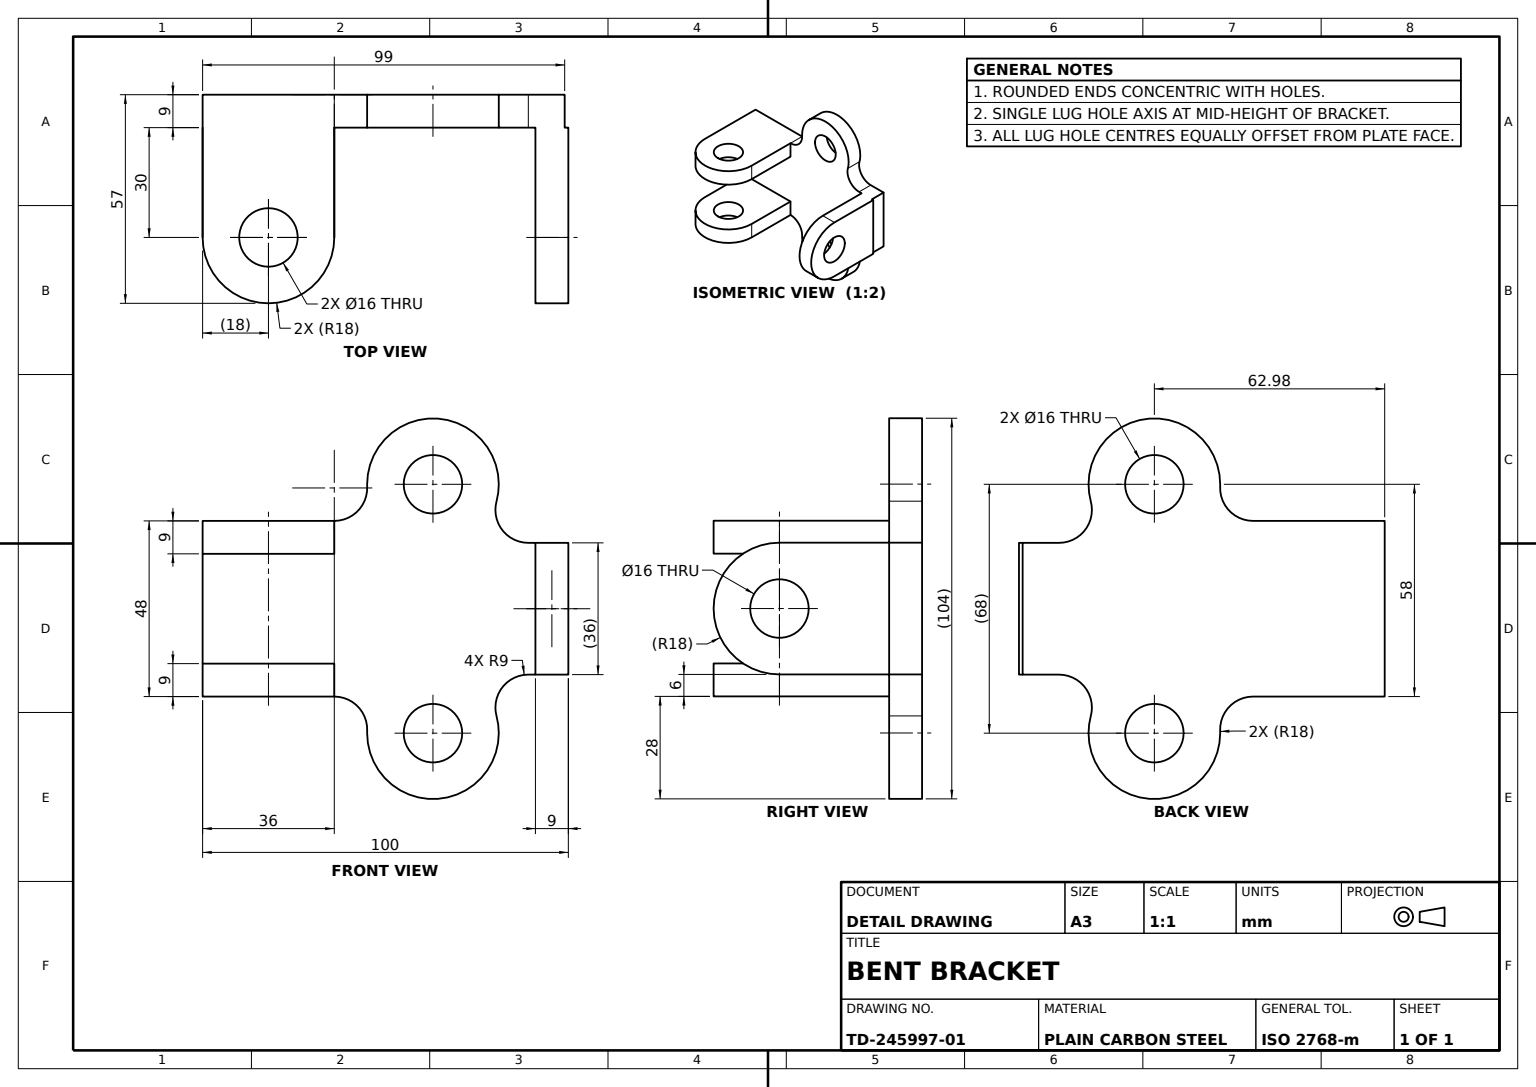
SolidWorks part; units mm, degrees
material "Plain Carbon Steel"
ref_plane "Front Plane" through (0, 0, 0) normal (0, 0, 1) x (1, 0, 0)
ref_plane "Top Plane" through (0, 0, 0) normal (0, 1, 0) x (1, 0, 0)
ref_plane "Right Plane" through (0, 0, 0) normal (1, 0, 0) x (0, 0, -1)
sketch "Base Plate Profile Sketch" plane through (0, 0, 0) normal (0, 0, 1) x (1, 0, 0)
  line L0 (0, 0) -> (0, 48)
  line L1 (0, 24) -> (62.9815, 24) construction
  line L2 (62.9815, 24) -> (99, 24) construction
  line L3 (99, 24) -> (99, 42)
  line L4 (99, 24) -> (99, 6)
  line L5 (62.9815, 24) -> (62.9815, 58) construction
  line L6 (62.9815, 24) -> (62.9815, -10) construction
  line L7 (0, 48) -> (36, 48)
  line L8 (99, 42) -> (89.0583, 42)
  line L9 (0, 0) -> (36, 0)
  line L10 (99, 6) -> (89.0583, 6)
  circle A0 centre (62.9815, 58) radius 8
  arc A1 (80.366, 53.3333) -> (44.9938, 57.3333) centre (62.9815, 58) ccw
  arc A2 (36, 48) -> (44.9938, 57.3333) centre (36, 57) ccw
  arc A3 (80.366, 53.3333) -> (89.0583, 42) centre (89.0583, 51) ccw
  circle A4 centre (62.9815, -10) radius 8
  arc A5 (44.9938, -9.3333) -> (80.366, -5.3333) centre (62.9815, -10) ccw
  arc A8 (44.9938, -9.3333) -> (36, 0) centre (36, -9) ccw
  arc A9 (89.0583, 6) -> (80.366, -5.3333) centre (89.0583, -3) ccw
  dimension "D1" = 16
  dimension "D2" = 36
  dimension "D3" = 48
  dimension "D7" = 9
  dimension "D8" = 58
  dimension "D10" = 9
  dimension "D11" = 99
  dimension "D12" = 16
  dimension "D13" = 18
  dimension "D14" = 9
  dimension "D4" = 18
  dimension "D15" = 18
  dimension "D5" = 36
  dimension "D6" = 68
  dimension "D9" = 18
extrude "Base Plate 9mm" add sketch "Base Plate Profile Sketch" along normal blind 9
ref_plane "Plane4" through (100, 0, 0) normal (1, 0, 0) x (0, 0, -1)
sketch "Lug Sketch X100" plane through (100, 0, 0) normal (1, 0, 0) x (0, 0, -1)
  line L0 (0, 6) -> (0, 42) construction
  line L1 (30, 42) -> (0, 42)
  line L2 (0, 42) -> (0, 6)
  line L3 (0, 6) -> (30, 6)
  circle A0 centre (30, 24) radius 8
  arc A1 (30, 6) -> (30, 42) centre (30, 24) ccw
  dimension "D1" = 30
  dimension "D2" = 36
  dimension "D3" = 16
extrude "Lug X100" add sketch "Lug Sketch X100" against normal blind 9
ref_plane "Plane5" through (0, 0, 0) normal (0, 1, 0) x (1, 0, 0)
sketch "Lug Sketch X0" plane through (0, 0, 0) normal (0, 1, 0) x (1, 0, 0)
  line L0 (36, 0) -> (0, 0) construction
  line L1 (0, 30) -> (0, 0)
  line L2 (0, 0) -> (36, 0)
  line L3 (36, 0) -> (36, 30)
  circle A0 centre (18, 30) radius 8
  arc A1 (36, 30) -> (0, 30) centre (18, 30) ccw
  dimension "D1" = 36
  dimension "D2" = 16
  dimension "D3" = 30
extrude "Lug X0" add sketch "Lug Sketch X0" along normal blind 9
ref_plane "Plane6" through (0, 48, 0) normal (0, 1, 0) x (1, 0, 0)
sketch "Lug Sketch Offset 48" plane through (0, 48, 0) normal (0, 1, 0) x (1, 0, 0)
  line L0 (0, 30) -> (0, 0)
  line L1 (0, 0) -> (36, 0)
  line L2 (36, 0) -> (36, 30)
  circle A0 centre (18, 30) radius 8
  arc A1 (36, 30) -> (0, 30) centre (18, 30) ccw
  dimension "D1" = 16
extrude "Lug Offset 48" add sketch "Lug Sketch Offset 48" against normal blind 9
